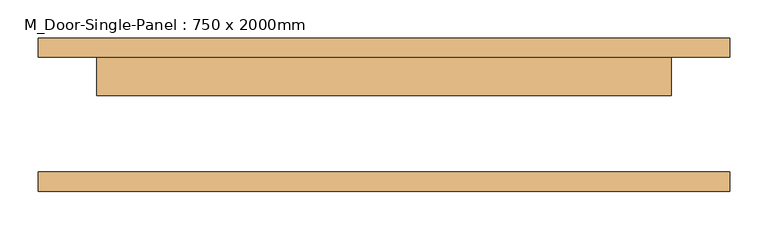
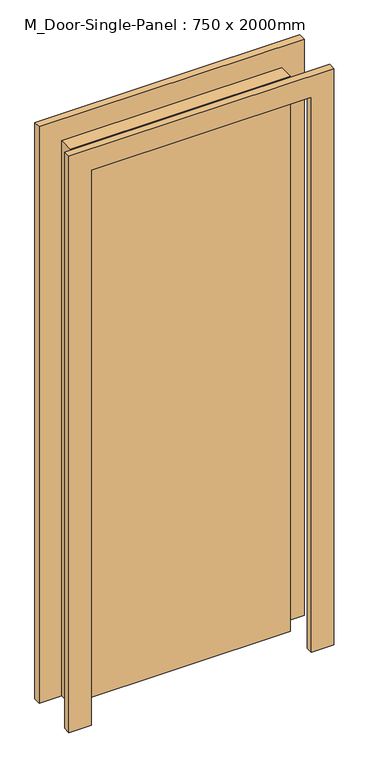
"""IFC4 building model written with IfcOpenShell, lengths in millimetres: door geometry, M_Door-Single-Panel : 750 x 2000mm."""

from ifc_helpers import new_model, si_unit, frame, origin, origin_with_axes, place, context, project, spatial, polyline, outline, extrude, source, transform, mapped, element, save


def m_door_single_panel_750_x_2000mm_5cf0dcc2(model_context):
    return source(origin(), model_context, "Body", "SweptSolid", [
        extrude(outline(polyline([(375.0, 25.0), (-375.0, 25.0), (-375.0, 75.0), (375.0, 75.0), (375.0, 25.0)])), origin_with_axes(), (0.0, 0.0, 1.0), 2000.0),
        extrude(outline(polyline([(2076.2, 451.2), (2076.2, -451.2), (0.0, -451.2), (0.0, -375.0), (2000.0, -375.0), (2000.0, 375.0), (0.0, 375.0), (0.0, 451.2), (2076.2, 451.2)])), frame((0.0, -100.0, 0.0), z_axis=(0.0, 1.0, 0.0), x_axis=(0.0, 0.0, 1.0)), (0.0, 0.0, 1.0), 25.0),
        extrude(outline(polyline([(2076.2, -451.2), (0.0, -451.2), (0.0, -375.0), (2000.0, -375.0), (2000.0, 375.0), (0.0, 375.0), (0.0, 451.2), (2076.2, 451.2), (2076.2, -451.2)])), frame((0.0, 75.0, 0.0), z_axis=(0.0, 1.0, 0.0), x_axis=(0.0, 0.0, 1.0)), (0.0, 0.0, 1.0), 25.0),
    ])


if __name__ == "__main__":
    model = new_model("IFC4")
    model_context = context("Model", 3, world=origin())
    ifc_project = project(units=[si_unit("LENGTHUNIT", "METRE", prefix="MILLI")], contexts=[model_context])
    site = spatial("IfcSite", under=ifc_project)
    building = spatial("IfcBuilding", under=site)
    placement = place(None, origin())
    m_door_single_panel_750_x_2000mm_shape = m_door_single_panel_750_x_2000mm_5cf0dcc2(model_context)
    element("IfcDoor", 1, ObjectType="M_Door-Single-Panel : 750 x 2000mm", at=placement, inside=building, context=model_context, shape_type="MappedRepresentation", body=[
        mapped(m_door_single_panel_750_x_2000mm_shape, transform((0.0, 0.0, 0.0), x_axis=(1.0, 0.0, 0.0), y_axis=(0.0, 1.0, 0.0), z_axis=(0.0, 0.0, 1.0))),
    ])
    save(model, "model.ifc")

# Revit data of these elements
# Type "M_Door-Single-Panel : 750 x 2000mm"
#   Type Mark = "42"
#   Construction Type Id = "DOOR"
#   Assembly Code = "C1020300"
#   Analytic Construction = "Wooden"
#   Thickness = 50 mm
#   Thermal Resistance (R) = 0.455703 (m²·K)/W
#   Swing Angle [instance default] = 90.00°
#   Heat Transfer Coefficient (U) = 2.19465 W/(m²·K)
#   Height = 2000 mm
#   Trim Projection Ext = 25 mm
#   Trim Projection Int = 25 mm
#   Trim Width = 80 mm
#   Width = 750 mm
#   Define Thermal Properties by = 1
#   Panel Material = Wood - Birch - Solid Stained Light Low Gloss
#   Trim Material = Paint - Sienna
#   Visual Light Transmittance = 0
#   Solar Heat Gain Coefficient = 0
#   Function = (empty or 0)
#   Wall Closure = (empty or 0)
# Element 1 (IfcDoor, "M_Door-Single-Panel : 750 x 2000mm")
#   Materials on its faces: "Paint - Sienna", "Wood - Birch - Solid Stained Light Low Gloss"
# Materials
#   "Wood - Birch - Solid Stained Light Low Gloss": class "Wood", colour RGB 210 159 95, transparency 0, Cost = 0
#   "Paint - Sienna": colour RGB 118 70 51, transparency 0, Cost = 0
